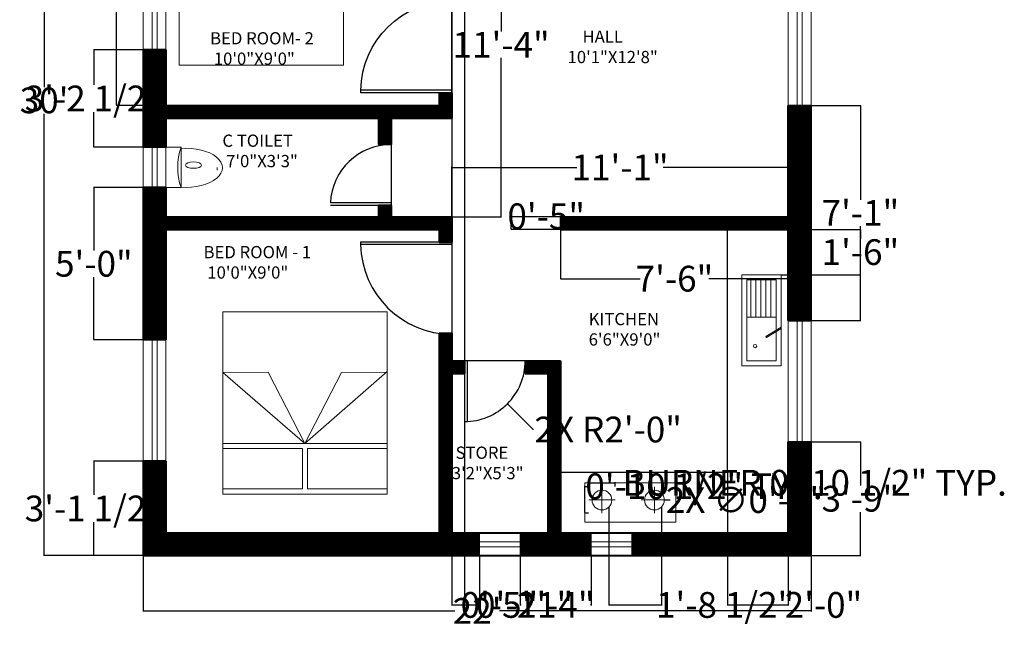
# Model space of a CAD drawing. Units: inches. Extents: x 254 to 1358, y 67 to 796.
# Tile 1 of 3: x 254 to 643, y 67 to 313. Entities that reach past the tile are written whole.
import ezdxf

# ---------------------------------------------------------------- set-up
doc = ezdxf.new("R2010")
doc.units = ezdxf.units.IN
doc.header["$MEASUREMENT"] = 0
for name, color, linetype, lineweight in [('A-ANNO-DIMS', 2, 'Continuous', 18), ('A-AREA-IDEN', 7, 'Continuous', 18), ('A-EQPM', 8, 'Continuous', 18), ('A-FLOR-CASE', 7, 'Continuous', 25), ('A-FLOR-FIXT', 9, 'Continuous', 18), ('A-FURN', 8, 'Continuous', 18), ('A-GLAZ', 160, 'Continuous', 18), ('A-WALL', 7, 'Continuous', 40), ('doors', 8, 'Continuous', 25)]:
    doc.layers.add(name, color=color, linetype=linetype, lineweight=lineweight)
doc.layers.add('A-WALL-PATT', color=251, linetype='Continuous', lineweight=13, true_color=0x636466)
doc.styles.get("Standard").update_dxf_attribs({"font": 'arial.ttf'})
doc.dimstyles.get("Standard").update_dxf_attribs({"dimtxt": 10.18, "dimasz": 0.18, "dimexe": 0.18, "dimexo": 0.0625, "dimgap": 0.09, "dimtad": 0, "dimtih": 1, "dimtoh": 1, "dimdec": 0, "dimzin": 0, "dimdsep": 46, "dimlunit": 3, "dimtxsty": 'Standard', "dimcen": 0.09, "dimadec": 0, "dimazin": 0, "dimtfac": 1, "dimtdec": 0, "dimtofl": 0, "dimtmove": 0, "dimatfit": 3, "dimfxl": 1, "dimtolj": 1, "dimtzin": 0, "dimarcsym": 0})

# ---------------------------------------------------------------- blocks, each defined once
blk = doc.blocks.new('*D4')
at = {"layer": 'A-ANNO-DIMS', "color": 0, "lineweight": -2, "transparency": 16777216}
for p, q in [((302.33, 461.54), (263.04, 461.54)), ((263.22, 461.36), (263.22, 286.83)), ((263.22, 101.72), (263.22, 276.25)), ((302.33, 101.54), (263.04, 101.54))]:
    blk.add_line(p, q, dxfattribs=at)
at = {"layer": 'A-ANNO-DIMS', "color": 0, "transparency": 16777216}
for points in [[(263.19, 461.36), (263.25, 461.36), (263.22, 461.54)], [(263.19, 101.72), (263.25, 101.72), (263.22, 101.54)]]:
    blk.add_solid(points, dxfattribs=at)
at = {"layer": 'Defpoints', "color": 0, "transparency": 16777216}
for p in [(302.39, 461.54), (263.22, 101.54), (302.39, 101.54)]:
    blk.add_point(p, dxfattribs=at)
at = {"layer": 'A-ANNO-DIMS', "color": 0, "transparency": 16777216, "insert": (263.22, 281.54), "char_height": 10.18, "attachment_point": 5}
blk.add_mtext("\\A1;30'", dxfattribs=at)
blk = doc.blocks.new('*D5')
at = {"layer": 'A-ANNO-DIMS', "color": 0, "lineweight": -2, "transparency": 16777216}
for p, q in [((302.39, 101.48), (302.39, 79.49)), ((566.39, 101.48), (566.39, 79.49)), ((302.57, 79.67), (425.58, 79.67)), ((566.21, 79.67), (443.21, 79.67))]:
    blk.add_line(p, q, dxfattribs=at)
at = {"layer": 'A-ANNO-DIMS', "color": 0, "transparency": 16777216}
for points in [[(302.57, 79.7), (302.57, 79.64), (302.39, 79.67)], [(566.21, 79.7), (566.21, 79.64), (566.39, 79.67)]]:
    blk.add_solid(points, dxfattribs=at)
at = {"layer": 'Defpoints', "color": 0, "transparency": 16777216}
for p in [(302.39, 101.54), (566.39, 101.54), (566.39, 79.67)]:
    blk.add_point(p, dxfattribs=at)
at = {"layer": 'A-ANNO-DIMS', "color": 0, "transparency": 16777216, "insert": (434.39, 79.67), "char_height": 10.18, "attachment_point": 5}
blk.add_mtext("\\A1;22'", dxfattribs=at)
blk = doc.blocks.new('WIN-48')
for p, q in [((9, 48), (0, 48)), ((0, 48), (0, 0)), ((3.5, 48), (3.5, 0)), ((5.5, 48), (5.5, 0)), ((5.5, 48), (5.5, 0)), ((5.5, 48), (5.5, 0)), ((5.5, 48), (5.5, 0)), ((9, 48), (9, 0)), ((9, 0), (0, 0))]:
    blk.add_line(p, q)
blk = doc.blocks.new('VENT-16')
for p, q in [((9, 16), (0, 16)), ((0, 16), (0, 0)), ((3.5, 16), (3.5, 0)), ((5.5, 16), (5.5, 0)), ((9, 16), (9, 0)), ((9, 0), (0, 0))]:
    blk.add_line(p, q)
blk = doc.blocks.new('DOOR-SWING-36')
for p, q in [((0, 0), (-36, 0)), ((-36, 0), (-36, -1)), ((0, 0), (0, -36.57)), ((0, -1), (-36, -1))]:
    blk.add_line(p, q)
blk.add_arc((0.31, -0.26), 36.31, 181.1696, 269.5155)
blk = doc.blocks.new('DOOR-SWING-24-BATH')
for p, q in [((0, 24), (0, 0)), ((0, 1), (-24, 1)), ((0, 0), (-24, 0))]:
    blk.add_line(p, q)
blk.add_arc((0, 0), 24, 90, 177.6141)
blk = doc.blocks.new('DOOR-SWING-24-INT')
for p, q in [((24, 0), (0, 0)), ((0, 0), (0, -24)), ((1, 0), (1, -24))]:
    blk.add_line(p, q)
blk.add_arc((0.03, -0.01), 23.97, 269.9169, 0.0334)
blk = doc.blocks.new('BED-DOUBLE')
for p, q in [((65, 72), (0, 72)), ((0, 72), (0, 0)), ((65, 0), (65, 72)), ((0, 48.04), (18, 48.19)), ((32.5, 20), (0, 48.04)), ((32.5, 20), (18, 48.19)), ((32.5, 20), (65, 48.44)), ((47, 48.04), (32.5, 20)), ((47, 48.04), (65, 48.19)), ((0, 20), (65, 20)), ((0, 18), (31.5, 18)), ((31.5, 18), (31.5, 2)), ((33.5, 18), (33.5, 2)), ((33.5, 18), (65, 18)), ((0, 2), (31.5, 2)), ((0, 0), (65, 0)), ((33.5, 2), (65, 2))]:
    blk.add_line(p, q)
blk = doc.blocks.new('WC-TANK')
for p, q in [((0, 8), (0, -8)), ((0, 8), (6, 8)), ((6, 8), (6, -8)), ((20.2, -1.04), (20.22, -0.04)), ((0, -8), (6, -8))]:
    blk.add_line(p, q)
blk.add_arc((29.23, 0), 24.57, 160.9964, 199.0036)
blk.add_ellipse((7.89, -0.16), major_axis=(14.43, 0), ratio=0.535102, start_param=4.576661, end_param=7.997223)
blk.add_ellipse((10.89, 0.89), major_axis=(3.17, 0), ratio=0.394417)
blk = doc.blocks.new('SINK-DRAINBOARD')
for p, q in [((15.54, 36), (0, 36)), ((0, 36), (0, 0)), ((15.54, 0), (15.54, 36)), ((13.54, 34), (2, 34)), ((2, 34), (2, 2)), ((3.54, 19.32), (3.54, 34)), ((5.54, 19.32), (5.54, 34)), ((7.54, 19.32), (7.54, 34)), ((9.54, 19.32), (9.54, 34)), ((11.54, 19.32), (11.54, 34)), ((13.54, 2), (13.54, 34)), ((13.54, 19.32), (2, 19.32)), ((15.54, 15.32), (9.48, 11.67)), ((9.73, 11.27), (15.54, 14.86)), ((11.54, 12.39), (11.54, 12.92)), ((9.48, 11.67), (9.73, 11.27)), ((0, 0), (15.54, 0)), ((2, 2), (13.54, 2))]:
    blk.add_line(p, q)
blk.add_circle((5.29, 7.86), 0.652)
blk = doc.blocks.new('COOKTOP-BURNER')
for p, q in [((0, -5.15), (0, 5.27)), ((5.21, 0.06), (-5.21, 0.06))]:
    blk.add_line(p, q)
blk.add_circle((0, 0), 3.91)
blk = doc.blocks.new('*D34')
at = {"layer": 'A-ANNO-DIMS', "color": 0, "lineweight": -2, "transparency": 16777216}
for p, q in [((478.52, 128.85), (478.52, 130.53)), ((478.7, 130.35), (488.75, 130.35)), ((488.93, 128.85), (488.93, 130.53)), ((488.93, 130.35), (489.11, 130.35))]:
    blk.add_line(p, q, dxfattribs=at)
at = {"layer": 'A-ANNO-DIMS', "color": 0, "transparency": 16777216}
for points in [[(478.7, 130.38), (478.7, 130.32), (478.52, 130.35)], [(488.75, 130.38), (488.75, 130.32), (488.93, 130.35)]]:
    blk.add_solid(points, dxfattribs=at)
at = {"layer": 'Defpoints', "color": 0, "transparency": 16777216}
for p in [(478.52, 128.79), (488.93, 130.35), (488.93, 128.79)]:
    blk.add_point(p, dxfattribs=at)
at = {"layer": 'A-ANNO-DIMS', "color": 0, "transparency": 16777216, "insert": (567.82, 130.35), "char_height": 10.18, "attachment_point": 5}
blk.add_mtext('\\A1;BURNER 0\'-10 1/2" TYP.', dxfattribs=at)
blk = doc.blocks.new('*D35')
at = {"layer": 'A-ANNO-DIMS', "color": 0, "lineweight": -2, "transparency": 16777216}
for p, q in [((478.45, 128.79), (476.77, 128.79)), ((476.95, 128.79), (476.95, 128.97)), ((476.95, 128.97), (477.13, 128.97)), ((476.95, 118.55), (476.95, 128.61)), ((478.45, 118.37), (476.77, 118.37))]:
    blk.add_line(p, q, dxfattribs=at)
at = {"layer": 'A-ANNO-DIMS', "color": 0, "transparency": 16777216}
for points in [[(476.92, 128.61), (476.98, 128.61), (476.95, 128.79)], [(476.92, 118.55), (476.98, 118.55), (476.95, 118.37)]]:
    blk.add_solid(points, dxfattribs=at)
at = {"layer": 'Defpoints', "color": 0, "transparency": 16777216}
for p in [(476.95, 128.79), (478.52, 128.79), (478.52, 118.37)]:
    blk.add_point(p, dxfattribs=at)
at = {"layer": 'A-ANNO-DIMS', "color": 0, "transparency": 16777216, "insert": (524.07, 128.97), "char_height": 10.18, "attachment_point": 5}
blk.add_mtext('\\A1;0\'-10 1/2" TYP.', dxfattribs=at)
blk = doc.blocks.new('*D36')
at = {"layer": 'A-ANNO-DIMS', "color": 0, "lineweight": -2, "transparency": 16777216}
for p, q in [((302.33, 138.84), (282.72, 138.84)), ((282.9, 138.66), (282.9, 125.55)), ((282.9, 101.72), (282.9, 114.83)), ((302.33, 101.54), (282.72, 101.54))]:
    blk.add_line(p, q, dxfattribs=at)
at = {"layer": 'A-ANNO-DIMS', "color": 0, "transparency": 16777216}
for points in [[(282.87, 138.66), (282.93, 138.66), (282.9, 138.84)], [(282.87, 101.72), (282.93, 101.72), (282.9, 101.54)]]:
    blk.add_solid(points, dxfattribs=at)
at = {"layer": 'Defpoints', "color": 0, "transparency": 16777216}
for p in [(282.9, 138.84), (302.39, 138.84), (302.39, 101.54)]:
    blk.add_point(p, dxfattribs=at)
at = {"layer": 'A-ANNO-DIMS', "color": 0, "transparency": 16777216, "insert": (282.9, 120.19), "char_height": 10.18, "attachment_point": 5}
blk.add_mtext('\\A1;3\'-1 1/2"', dxfattribs=at)
blk = doc.blocks.new('*D37')
at = {"layer": 'A-ANNO-DIMS', "color": 0, "lineweight": -2, "transparency": 16777216}
for p, q in [((302.33, 247.04), (282.72, 247.04)), ((282.9, 246.86), (282.9, 222.23)), ((282.9, 187.02), (282.9, 211.65)), ((302.33, 186.84), (282.72, 186.84))]:
    blk.add_line(p, q, dxfattribs=at)
at = {"layer": 'A-ANNO-DIMS', "color": 0, "transparency": 16777216}
for points in [[(282.87, 246.86), (282.93, 246.86), (282.9, 247.04)], [(282.87, 187.02), (282.93, 187.02), (282.9, 186.84)]]:
    blk.add_solid(points, dxfattribs=at)
at = {"layer": 'Defpoints', "color": 0, "transparency": 16777216}
for p in [(282.9, 247.04), (302.39, 247.04), (302.39, 186.84)]:
    blk.add_point(p, dxfattribs=at)
at = {"layer": 'A-ANNO-DIMS', "color": 0, "transparency": 16777216, "insert": (282.9, 216.94), "char_height": 10.18, "attachment_point": 5}
blk.add_mtext('\\A1;5\'-0"', dxfattribs=at)
blk = doc.blocks.new('*D38')
at = {"layer": 'A-ANNO-DIMS', "color": 0, "lineweight": -2, "transparency": 16777216}
for p, q in [((302.33, 301.54), (282.72, 301.54)), ((282.9, 301.36), (282.9, 287.65)), ((282.9, 263.22), (282.9, 276.94)), ((302.33, 263.04), (282.72, 263.04))]:
    blk.add_line(p, q, dxfattribs=at)
at = {"layer": 'A-ANNO-DIMS', "color": 0, "transparency": 16777216}
for points in [[(282.87, 301.36), (282.93, 301.36), (282.9, 301.54)], [(282.87, 263.22), (282.93, 263.22), (282.9, 263.04)]]:
    blk.add_solid(points, dxfattribs=at)
at = {"layer": 'Defpoints', "color": 0, "transparency": 16777216}
for p in [(282.9, 301.54), (302.39, 301.54), (302.39, 263.04)]:
    blk.add_point(p, dxfattribs=at)
at = {"layer": 'A-ANNO-DIMS', "color": 0, "transparency": 16777216, "insert": (282.9, 282.29), "char_height": 10.18, "attachment_point": 5}
blk.add_mtext('\\A1;3\'-2 1/2"', dxfattribs=at)
blk = doc.blocks.new('*D39')
at = {"layer": 'A-ANNO-DIMS', "color": 0, "lineweight": -2, "transparency": 16777216}
for p, q in [((566.46, 146.54), (586.06, 146.54)), ((585.88, 146.36), (585.88, 129.33)), ((585.88, 101.72), (585.88, 118.75)), ((566.46, 101.54), (586.06, 101.54))]:
    blk.add_line(p, q, dxfattribs=at)
at = {"layer": 'A-ANNO-DIMS', "color": 0, "transparency": 16777216}
for points in [[(585.85, 146.36), (585.91, 146.36), (585.88, 146.54)], [(585.85, 101.72), (585.91, 101.72), (585.88, 101.54)]]:
    blk.add_solid(points, dxfattribs=at)
at = {"layer": 'Defpoints', "color": 0, "transparency": 16777216}
for p in [(566.39, 146.54), (585.88, 146.54), (566.39, 101.54)]:
    blk.add_point(p, dxfattribs=at)
at = {"layer": 'A-ANNO-DIMS', "color": 0, "transparency": 16777216, "insert": (585.88, 124.04), "char_height": 10.18, "attachment_point": 5}
blk.add_mtext('\\A1;3\'-9"', dxfattribs=at)
blk = doc.blocks.new('*D40')
at = {"layer": 'A-ANNO-DIMS', "color": 0, "lineweight": -2, "transparency": 16777216}
for p, q in [((566.46, 279.54), (586.06, 279.54)), ((585.88, 279.36), (585.88, 242.24)), ((585.88, 194.72), (585.88, 231.84)), ((566.46, 194.54), (586.06, 194.54))]:
    blk.add_line(p, q, dxfattribs=at)
at = {"layer": 'A-ANNO-DIMS', "color": 0, "transparency": 16777216}
for points in [[(585.85, 279.36), (585.91, 279.36), (585.88, 279.54)], [(585.85, 194.72), (585.91, 194.72), (585.88, 194.54)]]:
    blk.add_solid(points, dxfattribs=at)
at = {"layer": 'Defpoints', "color": 0, "transparency": 16777216}
for p in [(566.39, 279.54), (585.88, 279.54), (566.39, 194.54)]:
    blk.add_point(p, dxfattribs=at)
at = {"layer": 'A-ANNO-DIMS', "color": 0, "transparency": 16777216, "insert": (585.88, 237.04), "char_height": 10.18, "attachment_point": 5}
blk.add_mtext('\\A1;7\'-1"', dxfattribs=at)
blk = doc.blocks.new('*D43')
at = {"layer": 'A-ANNO-DIMS', "color": 0, "lineweight": -2, "transparency": 16777216}
for p, q in [((424.39, 110.48), (424.39, 81.87)), ((435.39, 101.48), (435.39, 81.87)), ((424.57, 82.05), (435.21, 82.05)), ((435.39, 82.05), (435.57, 82.05))]:
    blk.add_line(p, q, dxfattribs=at)
at = {"layer": 'A-ANNO-DIMS', "color": 0, "transparency": 16777216}
for points in [[(424.57, 82.08), (424.57, 82.02), (424.39, 82.05)], [(435.21, 82.08), (435.21, 82.02), (435.39, 82.05)]]:
    blk.add_solid(points, dxfattribs=at)
at = {"layer": 'Defpoints', "color": 0, "transparency": 16777216}
for p in [(424.39, 110.54), (435.39, 101.54), (435.39, 82.05)]:
    blk.add_point(p, dxfattribs=at)
at = {"layer": 'A-ANNO-DIMS', "color": 0, "transparency": 16777216, "insert": (453.15, 82.05), "char_height": 10.18, "attachment_point": 5}
blk.add_mtext('\\A1;0\'-11"', dxfattribs=at)
blk = doc.blocks.new('*D44')
at = {"layer": 'A-ANNO-DIMS', "color": 0, "lineweight": -2, "transparency": 16777216}
for p, q in [((451.39, 101.48), (451.39, 81.87)), ((479.53, 101.48), (479.53, 81.87)), ((451.57, 82.05), (451.75, 82.05)), ((479.35, 82.05), (479.17, 82.05))]:
    blk.add_line(p, q, dxfattribs=at)
at = {"layer": 'A-ANNO-DIMS', "color": 0, "transparency": 16777216}
for points in [[(451.57, 82.08), (451.57, 82.02), (451.39, 82.05)], [(479.35, 82.08), (479.35, 82.02), (479.53, 82.05)]]:
    blk.add_solid(points, dxfattribs=at)
at = {"layer": 'Defpoints', "color": 0, "transparency": 16777216}
for p in [(451.39, 101.54), (479.53, 101.54), (479.53, 82.05)]:
    blk.add_point(p, dxfattribs=at)
at = {"layer": 'A-ANNO-DIMS', "color": 0, "transparency": 16777216, "insert": (465.46, 82.05), "char_height": 10.18, "attachment_point": 5}
blk.add_mtext('\\A1;2\'-4"', dxfattribs=at)
blk = doc.blocks.new('*D46')
at = {"layer": 'A-ANNO-DIMS', "color": 0, "lineweight": -2, "transparency": 16777216}
for p, q in [((467.33, 235.54), (447.72, 235.54)), ((447.9, 235.54), (447.9, 235.72)), ((447.9, 235.72), (448.08, 235.72)), ((447.9, 230.72), (447.9, 235.36)), ((467.33, 230.54), (447.72, 230.54))]:
    blk.add_line(p, q, dxfattribs=at)
at = {"layer": 'A-ANNO-DIMS', "color": 0, "transparency": 16777216}
for points in [[(447.87, 235.36), (447.93, 235.36), (447.9, 235.54)], [(447.87, 230.72), (447.93, 230.72), (447.9, 230.54)]]:
    blk.add_solid(points, dxfattribs=at)
at = {"layer": 'Defpoints', "color": 0, "transparency": 16777216}
for p in [(447.9, 235.54), (467.39, 235.54), (467.39, 230.54)]:
    blk.add_point(p, dxfattribs=at)
at = {"layer": 'A-ANNO-DIMS', "color": 0, "transparency": 16777216, "insert": (461.7, 235.72), "char_height": 10.18, "attachment_point": 5}
blk.add_mtext('\\A1;0\'-5"', dxfattribs=at)
blk = doc.blocks.new('*D47')
at = {"layer": 'A-ANNO-DIMS', "color": 0, "lineweight": -2, "transparency": 16777216}
for p, q in [((311.33, 371.54), (291.72, 371.54)), ((291.9, 371.36), (291.9, 330.83)), ((291.9, 279.72), (291.9, 320.26)), ((311.33, 279.54), (291.72, 279.54))]:
    blk.add_line(p, q, dxfattribs=at)
at = {"layer": 'A-ANNO-DIMS', "color": 0, "transparency": 16777216}
for points in [[(291.87, 371.36), (291.93, 371.36), (291.9, 371.54)], [(291.87, 279.72), (291.93, 279.72), (291.9, 279.54)]]:
    blk.add_solid(points, dxfattribs=at)
at = {"layer": 'Defpoints', "color": 0, "transparency": 16777216}
for p in [(291.9, 371.54), (311.39, 371.54), (311.39, 279.54)]:
    blk.add_point(p, dxfattribs=at)
at = {"layer": 'A-ANNO-DIMS', "color": 0, "transparency": 16777216, "insert": (291.9, 325.54), "char_height": 10.18, "attachment_point": 5}
blk.add_mtext('\\A1;7\'-8"', dxfattribs=at)
blk = doc.blocks.new('*D48')
at = {"layer": 'A-ANNO-DIMS', "color": 0, "lineweight": -2, "transparency": 16777216}
for p, q in [((424.39, 235.61), (424.39, 255.21)), ((424.57, 255.03), (473.8, 255.03)), ((557.21, 255.03), (507.99, 255.03)), ((557.39, 235.61), (557.39, 255.21))]:
    blk.add_line(p, q, dxfattribs=at)
at = {"layer": 'A-ANNO-DIMS', "color": 0, "transparency": 16777216}
for points in [[(424.57, 255.06), (424.57, 255), (424.39, 255.03)], [(557.21, 255.06), (557.21, 255), (557.39, 255.03)]]:
    blk.add_solid(points, dxfattribs=at)
at = {"layer": 'Defpoints', "color": 0, "transparency": 16777216}
for p in [(557.39, 255.03), (424.39, 235.54), (557.39, 235.54)]:
    blk.add_point(p, dxfattribs=at)
at = {"layer": 'A-ANNO-DIMS', "color": 0, "transparency": 16777216, "insert": (490.89, 255.03), "char_height": 10.18, "attachment_point": 5}
blk.add_mtext('\\A1;11\'-1"', dxfattribs=at)
blk = doc.blocks.new('*D49')
at = {"layer": 'A-ANNO-DIMS', "color": 0, "lineweight": -2, "transparency": 16777216}
for p, q in [((424.46, 371.54), (444.06, 371.54)), ((443.88, 371.36), (443.88, 308.74)), ((443.88, 235.72), (443.88, 298.34)), ((424.46, 235.54), (444.06, 235.54))]:
    blk.add_line(p, q, dxfattribs=at)
at = {"layer": 'A-ANNO-DIMS', "color": 0, "transparency": 16777216}
for points in [[(443.85, 371.36), (443.91, 371.36), (443.88, 371.54)], [(443.85, 235.72), (443.91, 235.72), (443.88, 235.54)]]:
    blk.add_solid(points, dxfattribs=at)
at = {"layer": 'Defpoints', "color": 0, "transparency": 16777216}
for p in [(424.39, 371.54), (424.39, 235.54), (443.88, 235.54)]:
    blk.add_point(p, dxfattribs=at)
at = {"layer": 'A-ANNO-DIMS', "color": 0, "transparency": 16777216, "insert": (443.88, 303.54), "char_height": 10.18, "attachment_point": 5}
blk.add_mtext('\\A1;11\'-4"', dxfattribs=at)
blk = doc.blocks.new('*D50')
at = {"layer": 'A-ANNO-DIMS', "color": 0, "lineweight": -2, "transparency": 16777216}
for p, q in [((467.39, 230.48), (467.39, 210.87)), ((557.39, 230.48), (557.39, 210.87)), ((467.57, 211.05), (498.81, 211.05)), ((557.21, 211.05), (525.97, 211.05))]:
    blk.add_line(p, q, dxfattribs=at)
at = {"layer": 'A-ANNO-DIMS', "color": 0, "transparency": 16777216}
for points in [[(467.57, 211.08), (467.57, 211.02), (467.39, 211.05)], [(557.21, 211.08), (557.21, 211.02), (557.39, 211.05)]]:
    blk.add_solid(points, dxfattribs=at)
at = {"layer": 'Defpoints', "color": 0, "transparency": 16777216}
for p in [(467.39, 230.54), (557.39, 230.54), (467.39, 211.05)]:
    blk.add_point(p, dxfattribs=at)
at = {"layer": 'A-ANNO-DIMS', "color": 0, "transparency": 16777216, "insert": (512.39, 211.05), "char_height": 10.18, "attachment_point": 5}
blk.add_mtext('\\A1;7\'-6"', dxfattribs=at)
blk = doc.blocks.new('*D51')
at = {"layer": 'A-ANNO-DIMS', "color": 0, "lineweight": -2, "transparency": 16777216}
for p, q in [((533.39, 134.48), (533.39, 81.87)), ((557.39, 110.48), (557.39, 81.87)), ((533.57, 82.05), (557.21, 82.05)), ((557.39, 82.05), (557.57, 82.05))]:
    blk.add_line(p, q, dxfattribs=at)
at = {"layer": 'A-ANNO-DIMS', "color": 0, "transparency": 16777216}
for points in [[(533.57, 82.08), (533.57, 82.02), (533.39, 82.05)], [(557.21, 82.08), (557.21, 82.02), (557.39, 82.05)]]:
    blk.add_solid(points, dxfattribs=at)
at = {"layer": 'Defpoints', "color": 0, "transparency": 16777216}
for p in [(533.39, 134.54), (557.39, 110.54), (557.39, 82.05)]:
    blk.add_point(p, dxfattribs=at)
at = {"layer": 'A-ANNO-DIMS', "color": 0, "transparency": 16777216, "insert": (571.28, 82.05), "char_height": 10.18, "attachment_point": 5}
blk.add_mtext('\\A1;2\'-0"', dxfattribs=at)
blk = doc.blocks.new('*D52')
at = {"layer": 'A-ANNO-DIMS', "color": 0, "lineweight": -2, "transparency": 16777216}
for p, q in [((486.49, 120.69), (486.49, 81.87)), ((507.23, 120.69), (507.23, 81.87)), ((486.67, 82.05), (507.05, 82.05)), ((507.23, 82.05), (507.41, 82.05))]:
    blk.add_line(p, q, dxfattribs=at)
at = {"layer": 'A-ANNO-DIMS', "color": 0, "transparency": 16777216}
for points in [[(486.67, 82.08), (486.67, 82.02), (486.49, 82.05)], [(507.05, 82.08), (507.05, 82.02), (507.23, 82.05)]]:
    blk.add_solid(points, dxfattribs=at)
at = {"layer": 'Defpoints', "color": 0, "transparency": 16777216}
for p in [(486.49, 120.75), (507.23, 120.75), (507.23, 82.05)]:
    blk.add_point(p, dxfattribs=at)
at = {"layer": 'A-ANNO-DIMS', "color": 0, "transparency": 16777216, "insert": (532.41, 82.05), "char_height": 10.18, "attachment_point": 5}
blk.add_mtext('\\A1;1\'-8 1/2"', dxfattribs=at)
blk = doc.blocks.new('*D53')
at = {"layer": 'A-ANNO-DIMS', "color": 0, "lineweight": -2, "transparency": 16777216}
for p, q in [((557.46, 230.54), (586.06, 230.54)), ((585.88, 230.36), (585.88, 226.83)), ((585.88, 212.72), (585.88, 216.26)), ((554.6, 212.54), (586.06, 212.54))]:
    blk.add_line(p, q, dxfattribs=at)
at = {"layer": 'A-ANNO-DIMS', "color": 0, "transparency": 16777216}
for points in [[(585.85, 230.36), (585.91, 230.36), (585.88, 230.54)], [(585.85, 212.72), (585.91, 212.72), (585.88, 212.54)]]:
    blk.add_solid(points, dxfattribs=at)
at = {"layer": 'Defpoints', "color": 0, "transparency": 16777216}
for p in [(557.39, 230.54), (554.54, 212.54), (585.88, 212.54)]:
    blk.add_point(p, dxfattribs=at)
at = {"layer": 'A-ANNO-DIMS', "color": 0, "transparency": 16777216, "insert": (585.88, 221.54), "char_height": 10.18, "attachment_point": 5}
blk.add_mtext('\\A1;1\'-6"', dxfattribs=at)
blk = doc.blocks.new('*D56')
at = {"layer": 'A-ANNO-DIMS', "color": 0, "lineweight": -2, "transparency": 16777216}
for p, q in [((429.39, 380.48), (429.39, 81.87)), ((424.39, 371.48), (424.39, 81.87)), ((424.57, 82.05), (429.21, 82.05)), ((429.39, 82.05), (429.57, 82.05))]:
    blk.add_line(p, q, dxfattribs=at)
at = {"layer": 'A-ANNO-DIMS', "color": 0, "transparency": 16777216}
for points in [[(424.57, 82.08), (424.57, 82.02), (424.39, 82.05)], [(429.21, 82.08), (429.21, 82.02), (429.39, 82.05)]]:
    blk.add_solid(points, dxfattribs=at)
at = {"layer": 'Defpoints', "color": 0, "transparency": 16777216}
for p in [(429.39, 380.54), (424.39, 371.54), (429.39, 82.05)]:
    blk.add_point(p, dxfattribs=at)
at = {"layer": 'A-ANNO-DIMS', "color": 0, "transparency": 16777216, "insert": (443.19, 82.05), "char_height": 10.18, "attachment_point": 5}
blk.add_mtext('\\A1;0\'-5"', dxfattribs=at)
blk = doc.blocks.new('*D59')
at = {"layer": 'A-ANNO-DIMS', "color": 0, "lineweight": -2, "transparency": 16777216}
for p, q in [((429.34, 178.53), (429.52, 178.53)), ((429.43, 178.44), (429.43, 178.62)), ((456.53, 151.4), (446.49, 161.45)), ((456.71, 151.4), (456.53, 151.4))]:
    blk.add_line(p, q, dxfattribs=at)
at = {"layer": 'A-ANNO-DIMS', "color": 0, "transparency": 16777216}
blk.add_solid([(446.51, 161.47), (446.47, 161.43), (446.37, 161.58)], dxfattribs=at)
at = {"layer": 'Defpoints', "color": 0, "transparency": 16777216}
for p in [(429.43, 178.53), (446.37, 161.58)]:
    blk.add_point(p, dxfattribs=at)
at = {"layer": 'A-ANNO-DIMS', "color": 0, "transparency": 16777216, "insert": (486.22, 151.4), "char_height": 10.18, "attachment_point": 5}
blk.add_mtext('\\A1;2X R2\'-0"', dxfattribs=at)
blk = doc.blocks.new('*D62')
at = {"layer": 'A-ANNO-DIMS', "color": 0, "lineweight": -2, "transparency": 16777216}
for p, q in [((504.37, 123.52), (504.55, 123.52)), ((504.46, 123.43), (504.46, 123.61)), ((510.72, 123.52), (508.56, 123.52))]:
    blk.add_line(p, q, dxfattribs=at)
at = {"layer": 'A-ANNO-DIMS', "color": 0, "transparency": 16777216}
blk.add_solid([(508.56, 123.55), (508.56, 123.49), (508.38, 123.52)], dxfattribs=at)
at = {"layer": 'Defpoints', "color": 0, "transparency": 16777216}
for p in [(500.55, 123.52), (508.38, 123.52)]:
    blk.add_point(p, dxfattribs=at)
at = {"layer": 'A-ANNO-DIMS', "color": 0, "transparency": 16777216, "insert": (540.63, 123.52), "char_height": 10.18, "attachment_point": 5}
blk.add_mtext('\\A1;2X ∅0\'-8"', dxfattribs=at)

msp = doc.modelspace()

# ---------------------------------------------------------------- hatches: boundary and pattern name
at = {"layer": 'A-WALL-PATT'}
h = msp.add_hatch(dxfattribs=at)
h.set_pattern_fill('ANSI31', color=256)
h.paths.add_polyline_path([(311.39, 452.54), (440.82, 452.54), (440.82, 461.54), (440.82, 461.54), (302.39, 461.54), (302.39, 349.54), (311.39, 349.54), (311.39, 371.54), (419.39, 371.54), (419.39, 320.73, -0.034566), (424.39, 321.12), (424.39, 371.54), (429.39, 371.54), (429.39, 380.54), (311.39, 380.54)])
h.paths.add_polyline_path([(424.39, 284.54), (419.39, 284.54), (419.39, 279.54), (311.39, 279.54), (311.39, 301.54), (302.39, 301.54), (302.39, 263.04), (311.39, 263.04), (311.39, 274.54), (395.39, 274.54), (395.39, 264.04), (400.39, 264.04), (400.39, 274.54), (424.39, 274.54)])
h.paths.add_polyline_path([(311.39, 230.54), (419.39, 230.54), (419.39, 225.54), (424.39, 225.54), (424.39, 235.54), (400.39, 235.54), (400.39, 240.04), (395.39, 240.04), (395.39, 235.54), (311.39, 235.54), (311.39, 247.04), (302.39, 247.04), (302.39, 186.84), (311.39, 186.84)])
h.paths.add_polyline_path([(311.39, 138.84), (302.39, 138.84), (302.39, 101.54), (435.39, 101.54), (435.39, 110.54), (424.39, 110.54), (424.39, 173.54), (429.39, 173.54), (429.39, 178.54), (424.39, 178.54), (424.39, 188.97, -0.034564), (419.39, 189.35), (419.39, 110.54), (311.39, 110.54)])
h.paths.add_polyline_path([(510.16, 461.54), (477.39, 461.54), (477.39, 452.54), (479.39, 452.54), (479.39, 380.54), (465.96, 380.54), (465.96, 371.54), (529.39, 371.54), (529.39, 380.54), (488.39, 380.54), (488.39, 452.54), (510.16, 452.54)])
h.paths.add_polyline_path([(566.39, 461.54), (542.27, 461.54), (542.27, 452.54), (557.39, 452.54), (557.39, 380.54), (553.39, 380.54), (553.39, 371.54), (557.39, 371.54), (557.39, 327.54), (566.39, 327.54)])
h.paths.add_polyline_path([(566.39, 279.54), (557.39, 279.54), (557.39, 235.54), (467.39, 235.54), (467.39, 230.54), (557.39, 230.54), (557.39, 194.54), (566.39, 194.54)])
h.paths.add_polyline_path([(566.39, 146.54), (557.39, 146.54), (557.39, 110.54), (495.53, 110.54), (495.53, 101.54), (566.39, 101.54)])
h.paths.add_polyline_path([(479.53, 110.54), (467.39, 110.54), (467.39, 178.54), (453.39, 178.54), (453.39, 173.54), (462.39, 173.54), (462.39, 110.54), (451.39, 110.54), (451.39, 101.54), (479.53, 101.54)])

# ---------------------------------------------------------------- linework, layer by layer
at = {"layer": 'A-EQPM'}
for p, q in [((476.92, 130.36), (476.92, 114.82)), ((512.92, 130.36), (476.92, 130.36)), ((512.92, 114.82), (512.92, 130.36)), ((476.92, 114.82), (512.92, 114.82))]:
    msp.add_line(p, q, dxfattribs=at)
at = {"layer": 'A-FLOR-CASE'}
for p, q in [((533.39, 134.54), (533.39, 230.54)), ((467.39, 134.54), (533.39, 134.54))]:
    msp.add_line(p, q, dxfattribs=at)
at = {"layer": 'A-WALL'}
for p, q in [((311.39, 301.54), (302.39, 301.54)), ((302.39, 301.54), (302.39, 263.04)), ((311.39, 301.54), (311.39, 279.54)), ((419.39, 284.54), (424.39, 284.54)), ((419.39, 284.54), (419.39, 279.54)), ((424.39, 284.54), (424.39, 274.54)), ((311.39, 279.54), (419.39, 279.54)), ((557.39, 235.54), (557.39, 279.54)), ((557.39, 279.54), (566.39, 279.54)), ((566.39, 194.54), (566.39, 279.54)), ((311.39, 274.54), (395.39, 274.54)), ((311.39, 274.54), (311.39, 263.04)), ((395.39, 274.54), (395.39, 264.04)), ((400.39, 274.54), (400.39, 264.04)), ((400.39, 274.54), (424.39, 274.54)), ((311.39, 263.04), (302.39, 263.04)), ((400.39, 264.04), (395.39, 264.04)), ((311.39, 247.04), (302.39, 247.04)), ((302.39, 247.04), (302.39, 186.84)), ((311.39, 247.04), (311.39, 235.54)), ((400.39, 240.04), (395.39, 240.04)), ((395.39, 240.04), (395.39, 235.54)), ((400.39, 240.04), (400.39, 235.54)), ((311.39, 235.54), (395.39, 235.54)), ((400.39, 235.54), (424.39, 235.54)), ((424.39, 235.54), (424.39, 225.54)), ((467.39, 235.54), (467.39, 230.54)), ((467.39, 235.54), (557.39, 235.54)), ((311.39, 230.54), (419.39, 230.54)), ((311.39, 230.54), (311.39, 186.84)), ((419.39, 230.54), (419.39, 225.54)), ((467.39, 230.54), (557.39, 230.54)), ((557.39, 194.54), (557.39, 230.54)), ((419.39, 225.54), (424.39, 225.54)), ((557.39, 194.54), (566.39, 194.54)), ((311.39, 186.84), (302.39, 186.84)), ((419.39, 189.54), (424.39, 189.54)), ((419.39, 189.54), (419.39, 110.54)), ((424.39, 189.54), (424.39, 178.54)), ((424.39, 178.54), (429.39, 178.54)), ((429.39, 178.54), (429.39, 173.54)), ((453.39, 178.54), (453.39, 173.54)), ((453.39, 178.54), (467.39, 178.54)), ((467.39, 178.54), (467.39, 110.54)), ((424.39, 173.54), (429.39, 173.54)), ((424.39, 173.54), (424.39, 110.54)), ((453.39, 173.54), (462.39, 173.54)), ((462.39, 173.54), (462.39, 110.54)), ((557.39, 110.54), (557.39, 146.54)), ((557.39, 146.54), (566.39, 146.54)), ((566.39, 101.54), (566.39, 146.54)), ((311.39, 138.84), (302.39, 138.84)), ((302.39, 138.84), (302.39, 101.54)), ((311.39, 138.84), (311.39, 110.54)), ((311.39, 110.54), (419.39, 110.54)), ((424.39, 110.54), (462.39, 110.54)), ((467.39, 110.54), (557.39, 110.54)), ((302.39, 101.54), (566.39, 101.54))]:
    msp.add_line(p, q, dxfattribs=at)

# ---------------------------------------------------------------- block references
at = {"layer": 'A-EQPM'}
for p in [(483.73, 123.52), (504.46, 123.52)]:
    msp.add_blockref('COOKTOP-BURNER', p, dxfattribs=at)
at = {"layer": 'A-FLOR-FIXT'}
for name, p in [('WC-TANK', (311.39, 255.04)), ('SINK-DRAINBOARD', (539, 176.54))]:
    msp.add_blockref(name, p, dxfattribs=at)
at = {"layer": 'A-FURN', "extrusion": (0, 0, -1), "zscale": -1, "rotation": 180}
msp.add_blockref('BED-DOUBLE', (-316.59, 367.42), dxfattribs=at)
at = {"layer": 'A-FURN'}
msp.add_blockref('BED-DOUBLE', (333.84, 125.89), dxfattribs=at)
at = {"layer": 'A-GLAZ'}
for name, p in [('WIN-48', (302.39, 301.54)), ('WIN-48', (557.39, 279.54)), ('VENT-16', (302.39, 247.04)), ('WIN-48', (557.39, 146.54)), ('WIN-48', (302.39, 138.84))]:
    msp.add_blockref(name, p, dxfattribs=at)
for p, rotation in [((451.39, 101.54), 90.00000000000021), ((495.53, 101.54), 90.00000000000003)]:
    msp.add_blockref('VENT-16', p, dxfattribs=dict(at, rotation=rotation))
at = {"layer": 'doors', "extrusion": (0, 0, -1), "zscale": -1, "rotation": 180}
msp.add_blockref('DOOR-SWING-36', (-424.39, 284.54), dxfattribs=at)
at = {"layer": 'doors'}
for name, p in [('DOOR-SWING-24-BATH', (400.39, 240.04)), ('DOOR-SWING-36', (424.35, 225.54)), ('DOOR-SWING-24-INT', (429.39, 178.54))]:
    msp.add_blockref(name, p, dxfattribs=at)

# ---------------------------------------------------------------- texts
at = {"layer": 'A-AREA-IDEN', "attachment_point": 1}
for s, insert, char_height in [('BED ROOM- 2\\P 10\'0"X9\'0"', (328.85, 308.51), 4.8351), ('    HALL  \\P10\'1"X12\'8"', (470.14, 309.16), 4.8351), ('C TOILET\\P 7\'0"X3\'3"', (333.71, 268.02), 4.835), ('BED ROOM - 1\\P 10\'0"X9\'0"', (326.27, 223.96), 4.8351), ('KITCHEN\\P6\'6"X9\'0"', (478.49, 197.49), 4.835), (' STORE\\P3\'2"X5\'3"', (424.39, 144.65), 4.835)]:
    msp.add_mtext_dynamic_manual_height_columns(s, width=48.103, gutter_width=24.18, heights=[18.78], dxfattribs=dict(at, insert=insert, char_height=char_height))

# ---------------------------------------------------------------- dimensions: what is measured, and where the dimension line sits
at = {"layer": 'A-ANNO-DIMS'}
for base, p1, p2, angle, override, picture, middle in [((263.22, 101.54), (302.39, 461.54), (302.39, 101.54), 90, {"dimclrd": 0, "dimclre": 0, "dimclrt": 0}, '*D4', (263.22, 281.54)), ((291.9, 371.54), (311.39, 279.54), (311.39, 371.54), 90, {"dimdec": 1, "dimlfac": 1, "dimrnd": 0, "dimzin": 1, "dimdsep": 46, "dimlunit": 4, "dimfrac": 2}, '*D47', (291.9, 325.54)), ((443.88, 235.54), (424.39, 371.54), (424.39, 235.54), 270, {"dimdec": 1, "dimlfac": 1, "dimrnd": 0, "dimzin": 1, "dimdsep": 46, "dimlunit": 4, "dimfrac": 2}, '*D49', (443.88, 303.54)), ((282.9, 301.54), (302.39, 263.04), (302.39, 301.54), 90, {"dimdec": 1, "dimlfac": 1, "dimrnd": 0, "dimzin": 1, "dimdsep": 46, "dimlunit": 4, "dimfrac": 2}, '*D38', (282.9, 282.29)), ((585.88, 279.54), (566.39, 194.54), (566.39, 279.54), 90, {"dimdec": 1, "dimlfac": 1, "dimrnd": 0, "dimzin": 1, "dimdsep": 46, "dimlunit": 4, "dimfrac": 2}, '*D40', (585.88, 237.04)), ((282.9, 247.04), (302.39, 186.84), (302.39, 247.04), 90, {"dimdec": 1, "dimlfac": 1, "dimrnd": 0, "dimzin": 1, "dimdsep": 46, "dimlunit": 4, "dimfrac": 2}, '*D37', (282.9, 216.94)), ((447.9, 235.54), (467.39, 230.54), (467.39, 235.54), 90, {"dimdec": 1, "dimlfac": 1, "dimrnd": 0, "dimzin": 1, "dimdsep": 46, "dimlunit": 4, "dimfrac": 2}, '*D46', (461.7, 235.72)), ((467.39, 211.05), (557.39, 230.54), (467.39, 230.54), 180, {"dimdec": 1, "dimlfac": 1, "dimrnd": 0, "dimzin": 1, "dimdsep": 46, "dimlunit": 4, "dimfrac": 2}, '*D50', (512.39, 211.05)), ((585.88, 212.54), (557.39, 230.54), (554.54, 212.54), 90, {"dimdec": 1, "dimlfac": 1, "dimrnd": 0, "dimzin": 1, "dimdsep": 46, "dimlunit": 4, "dimfrac": 2}, '*D53', (585.88, 221.54)), ((585.88, 146.54), (566.39, 101.54), (566.39, 146.54), 90, {"dimdec": 1, "dimlfac": 1, "dimrnd": 0, "dimzin": 1, "dimdsep": 46, "dimlunit": 4, "dimfrac": 2}, '*D39', (585.88, 124.04)), ((282.9, 138.84), (302.39, 101.54), (302.39, 138.84), 90, {"dimdec": 1, "dimlfac": 1, "dimrnd": 0, "dimzin": 1, "dimdsep": 46, "dimlunit": 4, "dimfrac": 2}, '*D36', (282.9, 120.19))]:
    dim = msp.add_linear_dim(base=base, p1=p1, p2=p2, angle=angle, dimstyle='Standard', override=override, dxfattribs=at)
    dim.commit()
    dim.dimension.update_dxf_attribs({"geometry": picture, "text_midpoint": middle})
for base, p1, p2, override, picture, middle in [((429.39, 82.05), (424.39, 371.54), (429.39, 380.54), {"dimdec": 1, "dimlfac": 1, "dimrnd": 0, "dimzin": 1, "dimdsep": 46, "dimlunit": 4, "dimfrac": 2}, '*D56', (443.19, 82.05)), ((557.39, 255.03), (424.39, 235.54), (557.39, 235.54), {"dimdec": 1, "dimlfac": 1, "dimrnd": 0, "dimzin": 1, "dimdsep": 46, "dimlunit": 4, "dimfrac": 2}, '*D48', (490.89, 255.03)), ((557.39, 82.05), (533.39, 134.54), (557.39, 110.54), {"dimdec": 1, "dimlfac": 1, "dimrnd": 0, "dimzin": 1, "dimdsep": 46, "dimlunit": 4, "dimfrac": 2}, '*D51', (571.28, 82.05)), ((507.23, 82.05), (486.49, 120.75), (507.23, 120.75), {"dimdec": 1, "dimlfac": 1, "dimrnd": 0, "dimzin": 1, "dimdsep": 46, "dimlunit": 4, "dimfrac": 2}, '*D52', (532.41, 82.05)), ((435.39, 82.05), (424.39, 110.54), (435.39, 101.54), {"dimdec": 1, "dimlfac": 1, "dimrnd": 0, "dimzin": 1, "dimdsep": 46, "dimlunit": 4, "dimfrac": 2}, '*D43', (453.15, 82.05)), ((566.39, 79.67), (302.39, 101.54), (566.39, 101.54), {"dimclrd": 0, "dimclre": 0, "dimclrt": 0}, '*D5', (434.39, 79.67)), ((479.53, 82.05), (451.39, 101.54), (479.53, 101.54), {"dimdec": 1, "dimlfac": 1, "dimrnd": 0, "dimzin": 1, "dimdsep": 46, "dimlunit": 4, "dimfrac": 2}, '*D44', (465.46, 82.05))]:
    dim = msp.add_linear_dim(base=base, p1=p1, p2=p2, dimstyle='Standard', override=override, dxfattribs=at)
    dim.commit()
    dim.dimension.update_dxf_attribs({"geometry": picture, "text_midpoint": middle})
dim = msp.add_radius_dim(center=(429.43, 178.53), mpoint=(446.37, 161.58), text='2X <>', dimstyle='Standard', override={"dimdec": 1, "dimlfac": 1, "dimrnd": 0, "dimzin": 1, "dimdsep": 46, "dimlunit": 4, "dimfrac": 2}, dxfattribs=at)
dim.commit()
dim.dimension.update_dxf_attribs({"geometry": '*D59', "text_midpoint": (486.22, 151.4), "dimtype": 164})
dim = msp.add_linear_dim(base=(488.93, 130.35), p1=(478.52, 128.79), p2=(488.93, 128.79), text='BURNER <> TYP.', dimstyle='Standard', override={"dimdec": 1, "dimlfac": 1, "dimrnd": 0, "dimzin": 1, "dimdsep": 46, "dimlunit": 4, "dimfrac": 2}, dxfattribs=at)
dim.commit()
dim.dimension.update_dxf_attribs({"geometry": '*D34', "text_midpoint": (567.82, 130.35)})
dim = msp.add_linear_dim(base=(476.95, 128.79), p1=(478.52, 118.37), p2=(478.52, 128.79), angle=90, text='<> TYP.', dimstyle='Standard', override={"dimdec": 1, "dimlfac": 1, "dimrnd": 0, "dimzin": 1, "dimdsep": 46, "dimlunit": 4, "dimfrac": 2}, dxfattribs=at)
dim.commit()
dim.dimension.update_dxf_attribs({"geometry": '*D35', "text_midpoint": (524.07, 128.97)})
dim = msp.add_diameter_dim_2p(p1=(500.55, 123.52), p2=(508.38, 123.52), text='2X <>', dimstyle='Standard', override={"dimdec": 1, "dimlfac": 1, "dimrnd": 0, "dimzin": 1, "dimdsep": 46, "dimlunit": 4, "dimfrac": 2}, dxfattribs=at)
dim.commit()
dim.dimension.update_dxf_attribs({"geometry": '*D62', "text_midpoint": (510.72, 123.52), "dimtype": 163})

doc.saveas('drawing.dxf')
